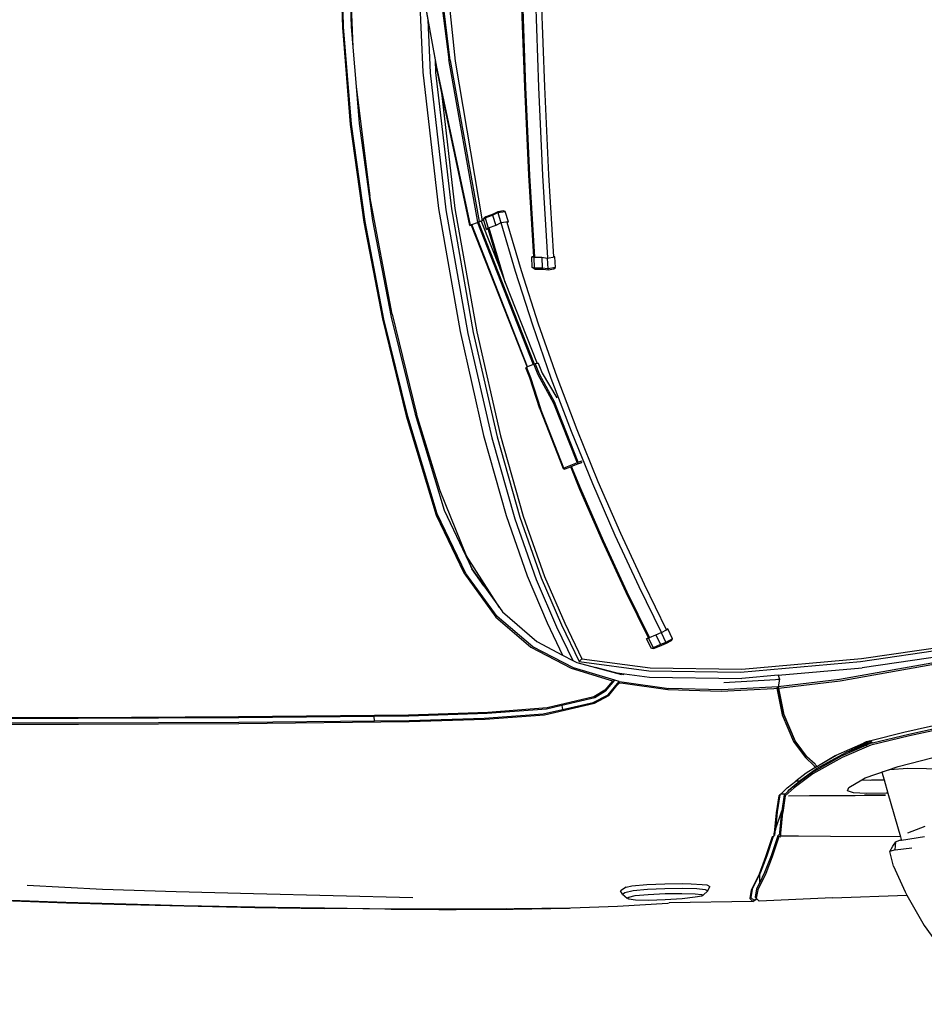
# Model space of a CAD drawing. Units: inches. Extents: x 22042254 to 25404563, y 17568978 to 17626777.
# Tile 11 of 45: x 22042340.9417 to 22042341.4576, y 17568977.6038 to 17568978.1657. Entities that reach past the tile are written whole.
import ezdxf

# ---------------------------------------------------------------- set-up
doc = ezdxf.new("R2010")
doc.units = ezdxf.units.IN
doc.header["$MEASUREMENT"] = 0
doc.layers.add('A-SITE-VEHI', color=8, linetype='Continuous', lineweight=18)
doc.layers.add('Edges', color=250, linetype='Continuous')

# ---------------------------------------------------------------- blocks, each defined once
blk = doc.blocks.new('Nissan Qashqai pl')
at = {"layer": 'Edges'}
for p, q in [((8.8066, 12.84004), (8.85915, 12.91267)), ((8.79082, 12.812), (8.8066, 12.84004)), ((8.19007, 12.82318), (8.1249, 12.82184)), ((8.12514, 12.82198), (8.19016, 12.82331)), ((8.20935, 12.82349), (8.19007, 12.82318)), ((8.19016, 12.82331), (8.25433, 12.82433)), ((8.25433, 12.82433), (8.20935, 12.82349)), ((8.25433, 12.8243), (8.20935, 12.82349)), ((8.25438, 12.8242), (8.20935, 12.82349)), ((8.26926, 12.82449), (8.25433, 12.82433)), ((8.31663, 12.82486), (8.25438, 12.8242)), ((8.31586, 12.82498), (8.26926, 12.82449)), ((8.30977, 12.82497), (8.26926, 12.82449)), ((8.31586, 12.82498), (8.30977, 12.82497)), ((8.31586, 12.82498), (8.31627, 12.82498)), ((8.31627, 12.82498), (8.35975, 12.8252)), ((8.31627, 12.82498), (8.36571, 12.82517)), ((8.37641, 12.82509), (8.31663, 12.82486)), ((8.35975, 12.8252), (8.36571, 12.82517)), ((8.36571, 12.82517), (8.36626, 12.82517)), ((8.36626, 12.82517), (8.3747, 12.8252)), ((8.37641, 12.82509), (8.36626, 12.82517)), ((8.3747, 12.8252), (8.37572, 12.8252)), ((8.37572, 12.8252), (8.4282, 12.82491)), ((8.40688, 12.82493), (8.37641, 12.82509)), ((8.42186, 12.82461), (8.40688, 12.82493)), ((8.42917, 12.82482), (8.40688, 12.82493)), ((8.4282, 12.82491), (8.47991, 12.82391)), ((8.47991, 12.82391), (8.42917, 12.82482)), ((8.47991, 12.82391), (8.48109, 12.82385)), ((8.48109, 12.82385), (8.52408, 12.82218)), ((8.01597, 12.81888), (7.96577, 12.81715)), ((7.96683, 12.81735), (8.01677, 12.81906)), ((8.07131, 12.82051), (8.01597, 12.81888)), ((8.01677, 12.81906), (8.07176, 12.82065)), ((8.1249, 12.82184), (8.07131, 12.82051)), ((8.07176, 12.82065), (8.12514, 12.82198)), ((8.26223, 12.81249), (8.33562, 12.8141)), ((8.52408, 12.82218), (8.5707, 12.81932)), ((8.52871, 12.81123), (8.5331, 12.81495)), ((8.53467, 12.81592), (8.5331, 12.81495)), ((8.5331, 12.81495), (8.53458, 12.81385)), ((8.53458, 12.81385), (8.54056, 12.81253)), ((8.54067, 12.81673), (8.53467, 12.81592)), ((8.55273, 12.81689), (8.54067, 12.81673)), ((8.56822, 12.81638), (8.55273, 12.81689)), ((8.58372, 12.81535), (8.56822, 12.81638)), ((8.5707, 12.81932), (8.57192, 12.81927)), ((8.64892, 12.81786), (8.57192, 12.81927)), ((8.59581, 12.81407), (8.58372, 12.81535)), ((8.6018, 12.81291), (8.59581, 12.81407)), ((8.64602, 12.81526), (8.64604, 12.81528)), ((8.64722, 12.80755), (8.64602, 12.81526)), ((8.64604, 12.81528), (8.64892, 12.81786)), ((8.64703, 12.81416), (8.64984, 12.81684)), ((8.64821, 12.8067), (8.64703, 12.81416)), ((8.64892, 12.81786), (8.65268, 12.81561)), ((8.64984, 12.81684), (8.65238, 12.81531)), ((8.65102, 12.814), (8.65204, 12.81496)), ((8.6524, 12.80636), (8.65102, 12.814)), ((8.65204, 12.81496), (8.65238, 12.81531)), ((8.65344, 12.80726), (8.65204, 12.81496)), ((8.65238, 12.81531), (8.65268, 12.81561)), ((8.65268, 12.81561), (8.65368, 12.81666)), ((8.65469, 12.81761), (8.65368, 12.81666)), ((8.65368, 12.81666), (8.65371, 12.81664)), ((8.7222, 12.8144), (8.65469, 12.81761)), ((8.7222, 12.8144), (8.79082, 12.812)), ((7.98032, 12.80297), (8.04999, 12.80661)), ((8.04999, 12.80661), (8.11758, 12.80867)), ((8.11758, 12.80867), (8.18881, 12.81066)), ((8.18881, 12.81066), (8.26223, 12.81249)), ((8.52871, 12.81123), (8.52689, 12.80817)), ((8.53223, 12.80475), (8.52689, 12.80817)), ((8.52871, 12.81123), (8.53103, 12.80953)), ((8.53103, 12.80953), (8.53854, 12.80786)), ((8.53223, 12.80475), (8.53747, 12.80359)), ((8.53854, 12.80786), (8.55176, 12.80664)), ((8.54056, 12.81253), (8.55262, 12.81139)), ((8.55176, 12.80664), (8.56796, 12.80592)), ((8.55262, 12.81139), (8.5681, 12.81066)), ((8.56796, 12.80592), (8.58417, 12.80574)), ((8.5681, 12.81066), (8.58359, 12.81044)), ((8.58359, 12.81044), (8.59567, 12.81073)), ((8.58417, 12.80574), (8.5974, 12.80608)), ((8.59567, 12.81073), (8.6017, 12.81139)), ((8.5974, 12.80608), (8.60494, 12.8069)), ((8.6017, 12.81139), (8.60325, 12.81209)), ((8.60325, 12.81209), (8.6018, 12.81291)), ((8.60732, 12.80799), (8.60325, 12.81209)), ((8.60494, 12.8069), (8.60732, 12.80799)), ((8.60732, 12.80799), (8.60927, 12.80397)), ((8.65464, 12.79258), (8.64722, 12.80755)), ((8.65502, 12.79287), (8.64821, 12.8067)), ((8.65502, 12.80099), (8.6524, 12.80636)), ((8.66083, 12.7921), (8.65344, 12.80726)), ((8.77849, 12.78548), (8.78905, 12.80886)), ((8.78905, 12.80886), (8.79082, 12.812)), ((8.53747, 12.80359), (8.55126, 12.80232)), ((8.55126, 12.80232), (8.56782, 12.8016)), ((8.56782, 12.8016), (8.58439, 12.80143)), ((8.58439, 12.80143), (8.5921, 12.80163)), ((8.5921, 12.80163), (8.60213, 12.80222)), ((8.60213, 12.80222), (8.6065, 12.80269)), ((8.6065, 12.80269), (8.60927, 12.80397)), ((8.65977, 12.79127), (8.65502, 12.80099)), ((8.65502, 12.79287), (8.65502, 12.80099)), ((8.66062, 12.77679), (8.65464, 12.79258)), ((8.65556, 12.79179), (8.65502, 12.79287)), ((8.65502, 12.79225), (8.65502, 12.79287)), ((8.66163, 12.77582), (8.65556, 12.79179)), ((8.66573, 12.77577), (8.65977, 12.79127)), ((8.66673, 12.77667), (8.66083, 12.7921)), ((8.77849, 12.78548), (8.77507, 12.77189)), ((8.66668, 12.75843), (8.66062, 12.77679)), ((8.66753, 12.75796), (8.66163, 12.77582)), ((8.67178, 12.75741), (8.66573, 12.77577)), ((8.67279, 12.75839), (8.66673, 12.77667)), ((8.77507, 12.77189), (8.7779, 12.76684)), ((8.77984, 12.77027), (8.77507, 12.77189)), ((8.77984, 12.77027), (8.78073, 12.76296)), ((8.77984, 12.77027), (8.7954, 12.76834)), ((8.7779, 12.76684), (8.78073, 12.76296)), ((8.78486, 12.7615), (8.78073, 12.76296)), ((8.78485, 12.75822), (8.7856, 12.7608)), ((8.78486, 12.7615), (8.78581, 12.76135)), ((8.78581, 12.76135), (8.7856, 12.7608)), ((8.78581, 12.76135), (8.80702, 12.75796)), ((8.66753, 12.75796), (8.66668, 12.75843)), ((8.6675, 12.75761), (8.66752, 12.75757)), ((8.66752, 12.75757), (8.66758, 12.75757)), ((8.66786, 12.75779), (8.66753, 12.75796)), ((8.66758, 12.75757), (8.66754, 12.75761)), ((8.66758, 12.75757), (8.66766, 12.75757)), ((8.66766, 12.75757), (8.66765, 12.7576)), ((8.66766, 12.75757), (8.66818, 12.75757)), ((8.66818, 12.75757), (8.66786, 12.75779)), ((8.66818, 12.75757), (8.66923, 12.75661)), ((8.66821, 12.75717), (8.66818, 12.75757)), ((8.66837, 12.75536), (8.66821, 12.75717)), ((8.66821, 12.75717), (8.66923, 12.75661)), ((8.66837, 12.75536), (8.66854, 12.75492)), ((8.6684, 12.755), (8.66837, 12.75536)), ((8.67032, 12.73608), (8.6684, 12.755)), ((8.66923, 12.75661), (8.6697, 12.75191)), ((8.6697, 12.75191), (8.6698, 12.75164)), ((8.67136, 12.73531), (8.6697, 12.75191)), ((8.6698, 12.75164), (8.67553, 12.7343)), ((8.67294, 12.7568), (8.67178, 12.75741)), ((8.67396, 12.7578), (8.67279, 12.75839)), ((8.67326, 12.75663), (8.67294, 12.7568)), ((8.67347, 12.75437), (8.67326, 12.75663)), ((8.67539, 12.73528), (8.67347, 12.75437)), ((8.67424, 12.7576), (8.67396, 12.7578)), ((8.67419, 12.75838), (8.67425, 12.75818)), ((8.67444, 12.75761), (8.67424, 12.7576)), ((8.67443, 12.75503), (8.67424, 12.7576)), ((8.67438, 12.7578), (8.67444, 12.75761)), ((8.67636, 12.736), (8.67443, 12.75503)), ((8.67726, 12.75766), (8.67444, 12.75761)), ((8.67908, 12.7578), (8.677, 12.75781)), ((8.6791, 12.75767), (8.67726, 12.75766)), ((8.72047, 12.75788), (8.67908, 12.7578)), ((8.6791, 12.75767), (8.67908, 12.7578)), ((8.68779, 12.75775), (8.67908, 12.7578)), ((8.68779, 12.75775), (8.6791, 12.75767)), ((8.68779, 12.75775), (8.68781, 12.75771)), ((8.69108, 12.75773), (8.68779, 12.75775)), ((8.72047, 12.75788), (8.69108, 12.75773)), ((8.78485, 12.75822), (8.72047, 12.75788)), ((8.77335, 12.71812), (8.78485, 12.75822)), ((8.79169, 12.7547), (8.80754, 12.74861)), ((8.67268, 12.72067), (8.67032, 12.73608)), ((8.6737, 12.7197), (8.67136, 12.73531)), ((8.67553, 12.7343), (8.67539, 12.73528)), ((8.67775, 12.71956), (8.67553, 12.7343)), ((8.67637, 12.7359), (8.67636, 12.736)), ((8.67876, 12.72047), (8.67637, 12.7359)), ((8.6737, 12.7197), (8.67268, 12.72067)), ((8.67458, 12.71886), (8.6737, 12.7197)), ((8.67852, 12.71886), (8.67458, 12.71886)), ((8.68052, 12.71323), (8.67458, 12.71886)), ((8.67852, 12.71886), (8.67775, 12.71956)), ((8.68152, 12.71616), (8.67852, 12.71886)), ((8.68699, 12.71316), (8.67876, 12.72047)), ((8.68152, 12.71616), (8.68177, 12.7154)), ((8.6817, 12.716), (8.68152, 12.71616)), ((8.6817, 12.716), (8.68177, 12.7154)), ((8.68592, 12.71219), (8.6817, 12.716)), ((8.68177, 12.7204), (8.70119, 12.72032)), ((8.68177, 12.7154), (8.69022, 12.70814)), ((8.70119, 12.72032), (8.70119, 12.72029)), ((8.70119, 12.72032), (8.70264, 12.72028)), ((8.70264, 12.72028), (8.70265, 12.72032)), ((8.70264, 12.72028), (8.70723, 12.72026)), ((8.70723, 12.72026), (8.70724, 12.7203)), ((8.70723, 12.72026), (8.72731, 12.72022)), ((8.72731, 12.72022), (8.7273, 12.72015)), ((8.72731, 12.72022), (8.73541, 12.72019)), ((8.7354, 12.72011), (8.73541, 12.72019)), ((8.73541, 12.72019), (8.74196, 12.72017)), ((8.74149, 12.7177), (8.73614, 12.71582)), ((8.73614, 12.71582), (8.73734, 12.71281)), ((8.75339, 12.71847), (8.74149, 12.7177)), ((8.74196, 12.72007), (8.74196, 12.72017)), ((8.74196, 12.72017), (8.74205, 12.72017)), ((8.74205, 12.72017), (8.74204, 12.72007)), ((8.74205, 12.72017), (8.74259, 12.72016)), ((8.74259, 12.72007), (8.74259, 12.72016)), ((8.74259, 12.72016), (8.74329, 12.72016)), ((8.74329, 12.72006), (8.74329, 12.72016)), ((8.74329, 12.72016), (8.77107, 12.72006)), ((8.77107, 12.72006), (8.75159, 12.72002)), ((8.77184, 12.71812), (8.75339, 12.71847)), ((8.76983, 12.70584), (8.77335, 12.71812)), ((8.77335, 12.71812), (8.77184, 12.71812)), ((8.68052, 12.71323), (8.68839, 12.70708)), ((8.69273, 12.70708), (8.68592, 12.71219)), ((8.70424, 12.7002), (8.68699, 12.71316)), ((8.69166, 12.70708), (8.68839, 12.70708)), ((8.69801, 12.69957), (8.68839, 12.70708)), ((8.69022, 12.70814), (8.69166, 12.70708)), ((8.69166, 12.70708), (8.70745, 12.69546)), ((8.69273, 12.70708), (8.69226, 12.70708)), ((8.70323, 12.69919), (8.69273, 12.70708)), ((8.73734, 12.71281), (8.74923, 12.70589)), ((8.74923, 12.70589), (8.75717, 12.70622)), ((8.74923, 12.70589), (8.75242, 12.70403)), ((8.75717, 12.70622), (8.76983, 12.70584)), ((8.76978, 12.70567), (8.75827, 12.70596)), ((8.76783, 12.69884), (8.76978, 12.70567)), ((8.76978, 12.70567), (8.76983, 12.70584)), ((8.70706, 12.69418), (8.69801, 12.69957)), ((8.73018, 12.68398), (8.70323, 12.69919)), ((8.73122, 12.68505), (8.70424, 12.7002)), ((8.75242, 12.70403), (8.78282, 12.69339)), ((8.77482, 12.6967), (8.76783, 12.69884)), ((8.79161, 12.69538), (8.77482, 12.6967)), ((8.82591, 12.6959), (8.79161, 12.69538)), ((8.69702, 12.685), (8.70548, 12.69273)), ((8.69793, 12.68388), (8.70617, 12.69146)), ((8.70617, 12.69146), (8.69867, 12.68446)), ((8.70548, 12.69273), (8.70706, 12.69418)), ((8.70617, 12.69146), (8.70675, 12.69195)), ((8.70675, 12.69195), (8.70829, 12.6934)), ((8.70706, 12.69418), (8.70829, 12.6934)), ((8.70745, 12.69546), (8.73458, 12.6806)), ((8.70832, 12.69343), (8.70829, 12.6934)), ((8.70832, 12.69338), (8.70829, 12.6934)), ((8.70832, 12.69338), (8.70832, 12.69343)), ((8.71019, 12.69229), (8.70832, 12.69338)), ((8.71021, 12.69228), (8.71019, 12.69229)), ((8.71084, 12.69191), (8.71021, 12.69228)), ((8.72567, 12.68326), (8.71084, 12.69191)), ((8.72477, 12.68364), (8.71084, 12.69191)), ((8.78282, 12.69339), (8.8245, 12.68281)), ((8.68642, 12.6706), (8.69702, 12.685)), ((8.68755, 12.66979), (8.69793, 12.68388)), ((8.69867, 12.68446), (8.69243, 12.67602)), ((8.72567, 12.68326), (8.72477, 12.68364)), ((8.72575, 12.6832), (8.72567, 12.68326)), ((8.72575, 12.6832), (8.75076, 12.67195)), ((8.75292, 12.67414), (8.73018, 12.68398)), ((8.75744, 12.67372), (8.73122, 12.68505)), ((8.73458, 12.6806), (8.74911, 12.67384)), ((8.73458, 12.6806), (8.75774, 12.67094)), ((8.67593, 12.64592), (8.68642, 12.6706)), ((8.67716, 12.64536), (8.68755, 12.66979)), ((8.68828, 12.67043), (8.67767, 12.64575)), ((8.69243, 12.67602), (8.68828, 12.67043)), ((8.69243, 12.67602), (8.69239, 12.67616)), ((8.75076, 12.67195), (8.74911, 12.67384)), ((8.74911, 12.67384), (8.7576, 12.66988)), ((8.75323, 12.67084), (8.75076, 12.67195)), ((8.75292, 12.67414), (8.75774, 12.67094)), ((8.75696, 12.67239), (8.75292, 12.67414)), ((8.75751, 12.66977), (8.75323, 12.67084)), ((8.75874, 12.67197), (8.75696, 12.67239)), ((8.79306, 12.6653), (8.75744, 12.67372)), ((8.7576, 12.66988), (8.75751, 12.66977)), ((8.7881, 12.66207), (8.75751, 12.66977)), ((8.75825, 12.67073), (8.7576, 12.66988)), ((8.75774, 12.67094), (8.75825, 12.67073)), ((8.75901, 12.6717), (8.75825, 12.67073)), ((8.75874, 12.67197), (8.75901, 12.6717)), ((8.75914, 12.67187), (8.75874, 12.67197)), ((8.75914, 12.67187), (8.75901, 12.6717)), ((8.79247, 12.66397), (8.75914, 12.67187)), ((8.89182, 12.63919), (8.7881, 12.66207)), ((8.89406, 12.64182), (8.79247, 12.66397)), ((8.8942, 12.64323), (8.79306, 12.6653)), ((7.90357, 12.65342), (8.0275, 12.6533)), ((7.90396, 12.65472), (8.02759, 12.65454)), ((8.0275, 12.6533), (8.17546, 12.6527)), ((8.02759, 12.65454), (8.17534, 12.65386)), ((8.17534, 12.65386), (8.33243, 12.65213)), ((8.17546, 12.6527), (8.30049, 12.65138)), ((8.30049, 12.65138), (8.30019, 12.64741)), ((8.30049, 12.65138), (8.33242, 12.65104)), ((8.33242, 12.65104), (8.40141, 12.64883)), ((8.33243, 12.65213), (8.40223, 12.64982)), ((8.02732, 12.64849), (7.90142, 12.64867)), ((8.02749, 12.64934), (7.90204, 12.64948)), ((8.17527, 12.64786), (8.02732, 12.64849)), ((8.17541, 12.64873), (8.02749, 12.64934)), ((8.33175, 12.64617), (8.17527, 12.64786)), ((8.30019, 12.64741), (8.17541, 12.64873)), ((8.33197, 12.64707), (8.30019, 12.64741)), ((8.40486, 12.64371), (8.33175, 12.64617)), ((8.40425, 12.64469), (8.33197, 12.64707)), ((8.40141, 12.64883), (8.45586, 12.64505)), ((8.40223, 12.64982), (8.45708, 12.64586)), ((8.45884, 12.64053), (8.40425, 12.64469)), ((8.45947, 12.63948), (8.40486, 12.64371)), ((8.45586, 12.64505), (8.47359, 12.64094)), ((8.45708, 12.64586), (8.50294, 12.635)), ((8.67156, 12.62423), (8.67593, 12.64592)), ((8.67716, 12.64536), (8.6721, 12.62009)), ((8.67767, 12.64575), (8.67272, 12.62129)), ((8.47287, 12.63723), (8.45884, 12.64053)), ((8.50247, 12.62935), (8.45947, 12.63948)), ((8.47287, 12.63723), (8.47359, 12.64094)), ((8.50324, 12.63009), (8.47287, 12.63723)), ((8.47359, 12.64094), (8.50181, 12.6344)), ((8.50181, 12.6344), (8.51552, 12.62739)), ((8.50294, 12.635), (8.51632, 12.62793)), ((8.51253, 12.62314), (8.50247, 12.62935)), ((8.5132, 12.62397), (8.50324, 12.63009)), ((8.51766, 12.61698), (8.51253, 12.62314)), ((8.5132, 12.62397), (8.52164, 12.61386)), ((8.51552, 12.62739), (8.5258, 12.61509)), ((8.51632, 12.62793), (8.52367, 12.61894)), ((8.57063, 12.62256), (8.61967, 12.62406)), ((8.61967, 12.62406), (8.66831, 12.62153)), ((8.67099, 12.62142), (8.67156, 12.62423)), ((8.51661, 12.61349), (8.51971, 12.61447)), ((8.51971, 12.61447), (8.51766, 12.61698)), ((8.51971, 12.61447), (8.52164, 12.61386)), ((8.5258, 12.61509), (8.52164, 12.61386)), ((8.52367, 12.61894), (8.52592, 12.61624)), ((8.52592, 12.61624), (8.5258, 12.61509)), ((8.5258, 12.61509), (8.5304, 12.61573)), ((8.52592, 12.61624), (8.52937, 12.61673)), ((8.52937, 12.61673), (8.57063, 12.62256)), ((8.5304, 12.61573), (8.53043, 12.61574)), ((8.53043, 12.61574), (8.57154, 12.62148)), ((8.62035, 12.62286), (8.57154, 12.62148)), ((8.62035, 12.62286), (8.62038, 12.62286)), ((8.6721, 12.62009), (8.62038, 12.62286)), ((8.62205, 12.61611), (8.66989, 12.61318)), ((8.66831, 12.62153), (8.67099, 12.62142)), ((8.67099, 12.62142), (8.6721, 12.62009)), ((8.67272, 12.62129), (8.6721, 12.62009)), ((8.67332, 12.61285), (8.6721, 12.62009)), ((8.72874, 12.61343), (8.6721, 12.62009)), ((8.67272, 12.62129), (8.67531, 12.621)), ((8.67531, 12.621), (8.72921, 12.61463)), ((8.72921, 12.61463), (8.86656, 12.59005)), ((8.48142, 12.60286), (8.51661, 12.61349)), ((8.52164, 12.61386), (8.48381, 12.60269)), ((8.48894, 12.59687), (8.55313, 12.60545)), ((8.50391, 12.60231), (8.52797, 12.60881)), ((8.52159, 12.60682), (8.50391, 12.60231)), ((8.52159, 12.60682), (8.5538, 12.61113)), ((8.53014, 12.60901), (8.52159, 12.60682)), ((8.55313, 12.60545), (8.6375, 12.60659)), ((8.5538, 12.61113), (8.63869, 12.61228)), ((8.6375, 12.60659), (8.74806, 12.59685)), ((8.6721, 12.60934), (8.63869, 12.61228)), ((8.66989, 12.61318), (8.6721, 12.61297)), ((8.6721, 12.61271), (8.6721, 12.61297)), ((8.6721, 12.61297), (8.67332, 12.61285)), ((8.6721, 12.60934), (8.67332, 12.61285)), ((8.6721, 12.60934), (8.74957, 12.60252)), ((8.86656, 12.58878), (8.72874, 12.61343)), ((8.44441, 12.58341), (8.48142, 12.60286)), ((8.48381, 12.60269), (8.44622, 12.58328)), ((8.47252, 12.56301), (8.48894, 12.59687)), ((8.48305, 12.59574), (8.48667, 12.59765)), ((8.48667, 12.59765), (8.50391, 12.60231)), ((8.49139, 12.59418), (8.48894, 12.59687)), ((8.49139, 12.59418), (8.55442, 12.6026)), ((8.55442, 12.6026), (8.63861, 12.60373)), ((8.63861, 12.60373), (8.74909, 12.59402)), ((8.74806, 12.59685), (8.87447, 12.5782)), ((8.87607, 12.58392), (8.74957, 12.60252)), ((8.44994, 12.57823), (8.47371, 12.5908)), ((8.45936, 12.56105), (8.47371, 12.5908)), ((8.46803, 12.56483), (8.48305, 12.59574)), ((8.47371, 12.5908), (8.48305, 12.59574)), ((8.47556, 12.56152), (8.49139, 12.59418)), ((8.74909, 12.59402), (8.87542, 12.5755)), ((8.41218, 12.55584), (8.44441, 12.58341)), ((8.44622, 12.58328), (8.41339, 12.55539)), ((8.41829, 12.55081), (8.44994, 12.57823)), ((8.5554, 12.58468), (8.55104, 12.57569)), ((8.55286, 12.57507), (8.55721, 12.58406)), ((8.55745, 12.58489), (8.5554, 12.58468)), ((8.55721, 12.58406), (8.5554, 12.58468)), ((8.56386, 12.58101), (8.55721, 12.58406)), ((8.55745, 12.58489), (8.55836, 12.58458)), ((8.55824, 12.58453), (8.55745, 12.58489)), ((8.55836, 12.58458), (8.56493, 12.58156)), ((8.55951, 12.57202), (8.56386, 12.58101)), ((8.56875, 12.57913), (8.56386, 12.58101)), ((8.56439, 12.57013), (8.56875, 12.57913)), ((8.56493, 12.58156), (8.56931, 12.57988)), ((8.56875, 12.57913), (8.56931, 12.57988)), ((8.57488, 12.57575), (8.56875, 12.57913)), ((8.56931, 12.57988), (8.57389, 12.57735)), ((8.55272, 12.57492), (8.53226, 12.53325)), ((8.55368, 12.57469), (8.53316, 12.53288)), ((8.56469, 12.56997), (8.54406, 12.52795)), ((8.55272, 12.57492), (8.55104, 12.57569)), ((8.55104, 12.57569), (8.5528, 12.57509)), ((8.5528, 12.57509), (8.55272, 12.57492)), ((8.5528, 12.57509), (8.55286, 12.57507)), ((8.55286, 12.57507), (8.55368, 12.57469)), ((8.55368, 12.57469), (8.55951, 12.57202)), ((8.55951, 12.57202), (8.56439, 12.57013)), ((8.56439, 12.57013), (8.56469, 12.56997)), ((8.56469, 12.56997), (8.56925, 12.56746)), ((8.57488, 12.57575), (8.57053, 12.56675)), ((8.57389, 12.57735), (8.57488, 12.57575)), ((8.44108, 12.51782), (8.45936, 12.56105)), ((8.44935, 12.52124), (8.46803, 12.56483)), ((8.45396, 12.51963), (8.47252, 12.56301)), ((8.45708, 12.51836), (8.47556, 12.56152)), ((8.54869, 12.52559), (8.5692, 12.56736)), ((8.5692, 12.56736), (8.56925, 12.56746)), ((8.57053, 12.56675), (8.5692, 12.56736)), ((8.56925, 12.56746), (8.57053, 12.56675)), ((8.3826, 12.51507), (8.41218, 12.55584)), ((8.41339, 12.55539), (8.38444, 12.51574)), ((8.41558, 12.54704), (8.41829, 12.55081)), ((8.41545, 12.54683), (8.38521, 12.49936)), ((8.39008, 12.51131), (8.41545, 12.54683)), ((8.40108, 12.52686), (8.41545, 12.54683)), ((8.41558, 12.54704), (8.41545, 12.54683)), ((8.53226, 12.53325), (8.51034, 12.48594)), ((8.53316, 12.53288), (8.51123, 12.48555)), ((8.40108, 12.52686), (8.39008, 12.51131)), ((8.39041, 12.51201), (8.40108, 12.52686)), ((8.54406, 12.52795), (8.52216, 12.48069)), ((8.52689, 12.47854), (8.54869, 12.52559)), ((8.35734, 12.46178), (8.3826, 12.51507)), ((8.38444, 12.51574), (8.3582, 12.46056)), ((8.42173, 12.46216), (8.44108, 12.51782)), ((8.42956, 12.4651), (8.44935, 12.52124)), ((8.43429, 12.46374), (8.45396, 12.51963)), ((8.43748, 12.46269), (8.45708, 12.51836)), ((8.36461, 12.45718), (8.38997, 12.51108)), ((8.36476, 12.45788), (8.38997, 12.51108)), ((8.38997, 12.51108), (8.38521, 12.49936)), ((8.38997, 12.51108), (8.39008, 12.51131)), ((8.39008, 12.51131), (8.39041, 12.51201)), ((8.38521, 12.49936), (8.36083, 12.43935)), ((8.51034, 12.48594), (8.48951, 12.43811)), ((8.51123, 12.48555), (8.49039, 12.4377)), ((8.52216, 12.48069), (8.50136, 12.43291)), ((8.50618, 12.43097), (8.52689, 12.47854)), ((8.32965, 12.37027), (8.35734, 12.46178)), ((8.3582, 12.46056), (8.33108, 12.37081)), ((8.40094, 12.3883), (8.42173, 12.46216)), ((8.40842, 12.39071), (8.42956, 12.4651)), ((8.41325, 12.38959), (8.43429, 12.46374)), ((8.41649, 12.38876), (8.43748, 12.46269)), ((8.33775, 12.36888), (8.36461, 12.45718)), ((8.36461, 12.45718), (8.36475, 12.45786)), ((8.36475, 12.45786), (8.36476, 12.45788)), ((8.36082, 12.43932), (8.33915, 12.3684)), ((8.36082, 12.43932), (8.36083, 12.43935)), ((8.48951, 12.43811), (8.48109, 12.41743)), ((8.50136, 12.43291), (8.48171, 12.38466)), ((8.49039, 12.4377), (8.48199, 12.41707)), ((8.48662, 12.38294), (8.50618, 12.43097)), ((8.45263, 12.36389), (8.47421, 12.41877)), ((8.47475, 12.41851), (8.45317, 12.36363)), ((8.47421, 12.41877), (8.47544, 12.41935)), ((8.47475, 12.41851), (8.47421, 12.41877)), ((8.47544, 12.41935), (8.47475, 12.41851)), ((8.48694, 12.41357), (8.47475, 12.41851)), ((8.47544, 12.41935), (8.48763, 12.4144)), ((8.47906, 12.41826), (8.47544, 12.41935)), ((8.48109, 12.41743), (8.47906, 12.41826)), ((8.48199, 12.41707), (8.48109, 12.41743)), ((8.49125, 12.41331), (8.48199, 12.41707)), ((8.48694, 12.41357), (8.48763, 12.4144)), ((8.48763, 12.4144), (8.49125, 12.41331)), ((8.48763, 12.4144), (8.48814, 12.41311)), ((8.46536, 12.35868), (8.48694, 12.41357)), ((8.48814, 12.41311), (8.46656, 12.35823)), ((8.48814, 12.41311), (8.48694, 12.41357)), ((8.49138, 12.41214), (8.48814, 12.41311)), ((8.49128, 12.41329), (8.49125, 12.41331)), ((8.49128, 12.41322), (8.49128, 12.41329)), ((8.37916, 12.29262), (8.40094, 12.3883)), ((8.38635, 12.29445), (8.40842, 12.39071)), ((8.39129, 12.29354), (8.41325, 12.38959)), ((8.39454, 12.29289), (8.41649, 12.38876)), ((8.48171, 12.38466), (8.46327, 12.33594)), ((8.46826, 12.33445), (8.48662, 12.38294)), ((8.30764, 12.28101), (8.32965, 12.37027)), ((8.33108, 12.37081), (8.3089, 12.28107)), ((8.31566, 12.2795), (8.33775, 12.36888)), ((8.31658, 12.27668), (8.33915, 12.3684)), ((8.45263, 12.36389), (8.44339, 12.33527)), ((8.44394, 12.33502), (8.45317, 12.36363)), ((8.4509, 12.33219), (8.46536, 12.35868)), ((8.4521, 12.33174), (8.46656, 12.35823)), ((8.45473, 12.33095), (8.46822, 12.35383)), ((8.44339, 12.33527), (8.43974, 12.32597)), ((8.44028, 12.32572), (8.44394, 12.33502)), ((8.46327, 12.33594), (8.44609, 12.28682)), ((8.45115, 12.28557), (8.46826, 12.33445)), ((8.38939, 12.19444), (8.44091, 12.32546)), ((8.44147, 12.32523), (8.3899, 12.1941)), ((8.44028, 12.32572), (8.43974, 12.32597)), ((8.44091, 12.32546), (8.44028, 12.32572)), ((8.44147, 12.32523), (8.44091, 12.32546)), ((8.44669, 12.32311), (8.44147, 12.32523)), ((8.44724, 12.32289), (8.4509, 12.33219)), ((8.44844, 12.32244), (8.4521, 12.33174)), ((8.45107, 12.32165), (8.45473, 12.33095)), ((8.39513, 12.19198), (8.44669, 12.32311)), ((8.44788, 12.32265), (8.39633, 12.19153)), ((8.4209, 12.24749), (8.45017, 12.32192)), ((8.44724, 12.32289), (8.44669, 12.32311)), ((8.44788, 12.32265), (8.44724, 12.32289)), ((8.44844, 12.32244), (8.44788, 12.32265)), ((8.45017, 12.32192), (8.44844, 12.32244)), ((8.45107, 12.32165), (8.45017, 12.32192)), ((8.35927, 12.17908), (8.37916, 12.29262)), ((8.36623, 12.1803), (8.38635, 12.29445)), ((8.37126, 12.17963), (8.39129, 12.29354)), ((8.37452, 12.17917), (8.39454, 12.29289)), ((8.29048, 12.19179), (8.30764, 12.28101)), ((8.3089, 12.28107), (8.29164, 12.19132)), ((8.2985, 12.19013), (8.31566, 12.2795)), ((8.44609, 12.28682), (8.43021, 12.23731)), ((8.43534, 12.2363), (8.45115, 12.28557)), ((8.31658, 12.27668), (8.29596, 12.16799)), ((8.41634, 12.23589), (8.4209, 12.24749)), ((8.4209, 12.24749), (8.41908, 12.2418)), ((8.39863, 12.19084), (8.41634, 12.23589)), ((8.41634, 12.23589), (8.40524, 12.19794)), ((8.41908, 12.2418), (8.40606, 12.19727)), ((8.43021, 12.23731), (8.41715, 12.19257)), ((8.42236, 12.19188), (8.43534, 12.2363)), ((8.44571, 12.23369), (8.44521, 12.22375)), ((8.4475, 12.23479), (8.44571, 12.23369)), ((8.44759, 12.23413), (8.44571, 12.23369)), ((8.4471, 12.22419), (8.44759, 12.23413)), ((8.4475, 12.23479), (8.44844, 12.23501)), ((8.45546, 12.23478), (8.4475, 12.23479)), ((8.45487, 12.23412), (8.44759, 12.23413)), ((8.44844, 12.23501), (8.45565, 12.235)), ((8.45438, 12.22418), (8.45487, 12.23412)), ((8.46004, 12.23485), (8.45487, 12.23412)), ((8.45565, 12.235), (8.46028, 12.23565)), ((8.45955, 12.22491), (8.46004, 12.23485)), ((8.46004, 12.23485), (8.46028, 12.23565)), ((8.46706, 12.23366), (8.46004, 12.23485)), ((8.46028, 12.23565), (8.46552, 12.23476)), ((8.46552, 12.23476), (8.46706, 12.23366)), ((8.46706, 12.23366), (8.46657, 12.22372)), ((8.44805, 12.22408), (8.44352, 12.14865)), ((8.44521, 12.22375), (8.4471, 12.22419)), ((8.44707, 12.22387), (8.44706, 12.22375)), ((8.4471, 12.22419), (8.45438, 12.22418)), ((8.45438, 12.22418), (8.45955, 12.22491)), ((8.46007, 12.2247), (8.45551, 12.14879)), ((8.45955, 12.22491), (8.46657, 12.22372)), ((8.46522, 12.22372), (8.46522, 12.22381)), ((8.44706, 12.22375), (8.44255, 12.14854)), ((8.44706, 12.22375), (8.44521, 12.22375)), ((8.46067, 12.1481), (8.46522, 12.22372)), ((8.46657, 12.22372), (8.46522, 12.22372)), ((8.40349, 12.19856), (8.40067, 12.18903)), ((8.40233, 12.18792), (8.40515, 12.19745)), ((8.40515, 12.19745), (8.40349, 12.19856)), ((8.40349, 12.19856), (8.40524, 12.19794)), ((8.41205, 12.19501), (8.40515, 12.19745)), ((8.40524, 12.19794), (8.40521, 12.19782)), ((8.2781, 12.10184), (8.29048, 12.19179)), ((8.29164, 12.19132), (8.27932, 12.10157)), ((8.28622, 12.10078), (8.2985, 12.19013)), ((8.38871, 12.19456), (8.35747, 12.04752)), ((8.38816, 12.19481), (8.36183, 12.06999)), ((8.39567, 12.19173), (8.36877, 12.04191)), ((8.37023, 12.0427), (8.39687, 12.19128)), ((8.37461, 12.04353), (8.3995, 12.19049)), ((8.38871, 12.19456), (8.38816, 12.19481)), ((8.38816, 12.19481), (8.38939, 12.19444)), ((8.38936, 12.19436), (8.38871, 12.19456)), ((8.38936, 12.19436), (8.38939, 12.19444)), ((8.38936, 12.19436), (8.3899, 12.1941)), ((8.3899, 12.1941), (8.39513, 12.19198)), ((8.39513, 12.19198), (8.39633, 12.19153)), ((8.39567, 12.19173), (8.39513, 12.19198)), ((8.39687, 12.19128), (8.39567, 12.19173)), ((8.39633, 12.19153), (8.39863, 12.19084)), ((8.3995, 12.19049), (8.39687, 12.19128)), ((8.3995, 12.19049), (8.39863, 12.19084)), ((8.40067, 12.18903), (8.40233, 12.18792)), ((8.40067, 12.18903), (8.40201, 12.18737)), ((8.40233, 12.18792), (8.40923, 12.18548)), ((8.40923, 12.18548), (8.41205, 12.19501)), ((8.41674, 12.19248), (8.41205, 12.19501)), ((8.41391, 12.18295), (8.41674, 12.19248)), ((8.42371, 12.1914), (8.41674, 12.19248)), ((8.42371, 12.1914), (8.42089, 12.18187)), ((8.42233, 12.19178), (8.42236, 12.19188)), ((8.42236, 12.19188), (8.42371, 12.1914)), ((8.34476, 12.05358), (8.35927, 12.17908)), ((8.35156, 12.05419), (8.36623, 12.1803)), ((8.35665, 12.05382), (8.37126, 12.17963)), ((8.36183, 12.06999), (8.37452, 12.17917)), ((8.40284, 12.18682), (8.40201, 12.18737)), ((8.40201, 12.18737), (8.4027, 12.18713)), ((8.40967, 12.1844), (8.40284, 12.18682)), ((8.40923, 12.18548), (8.41391, 12.18295)), ((8.41386, 12.18214), (8.40967, 12.1844)), ((8.41386, 12.18214), (8.41391, 12.18295)), ((8.41908, 12.18133), (8.41386, 12.18214)), ((8.41391, 12.18295), (8.42089, 12.18187)), ((8.42089, 12.18187), (8.41908, 12.18133)), ((8.2834, 12.06686), (8.29596, 12.16799)), ((8.44255, 12.14854), (8.43872, 12.06738)), ((8.44352, 12.14865), (8.43969, 12.06744)), ((8.45551, 12.14879), (8.45166, 12.06738)), ((8.45684, 12.06694), (8.46067, 12.1481)), ((8.27079, 12.01226), (8.2781, 12.10184)), ((8.27932, 12.10157), (8.27192, 12.01183)), ((8.2834, 12.06686), (8.28622, 12.10078)), ((8.36183, 12.06999), (8.35738, 12.04888)), ((8.28039, 12.03052), (8.2834, 12.06686)), ((8.43872, 12.06738), (8.43593, 11.9861)), ((8.43969, 12.06744), (8.4369, 11.98609)), ((8.45166, 12.06738), (8.44886, 11.98585)), ((8.45405, 11.98566), (8.45684, 12.06694)), ((8.34061, 11.95665), (8.34476, 12.05358)), ((8.34946, 12.00531), (8.35156, 12.05419)), ((8.35615, 12.04214), (8.35665, 12.05382)), ((8.35747, 12.04752), (8.31037, 11.78808)), ((8.37023, 12.0427), (8.33738, 11.78256)), ((8.35615, 12.04214), (8.35738, 12.04888)), ((8.35648, 11.87066), (8.37461, 12.04353)), ((8.33603, 11.78277), (8.36877, 12.04191)), ((8.34946, 12.00531), (8.35615, 12.04214)), ((8.27648, 11.92734), (8.28039, 12.03052)), ((8.27881, 12.01143), (8.28039, 12.03052)), ((8.26824, 11.92208), (8.27079, 12.01226)), ((8.27192, 12.01183), (8.26946, 11.92208)), ((8.27648, 11.92734), (8.27881, 12.01143)), ((8.34061, 11.95665), (8.34946, 12.00531))]:
    blk.add_line(p, q, dxfattribs=at)
blk = doc.blocks.new('CAR')
blk.add_blockref('Nissan Qashqai pl', (-9.74328, -11.91512))

msp = doc.modelspace()

# ---------------------------------------------------------------- block references
at = {"layer": 'A-SITE-VEHI', "xscale": -0.6191396643141144, "yscale": 0.6191396643141144, "zscale": 0.6191396643141144, "rotation": 180}
msp.add_blockref('CAR', (22042342.03736, 17568978.22147), dxfattribs=at)

doc.saveas('drawing.dxf')
